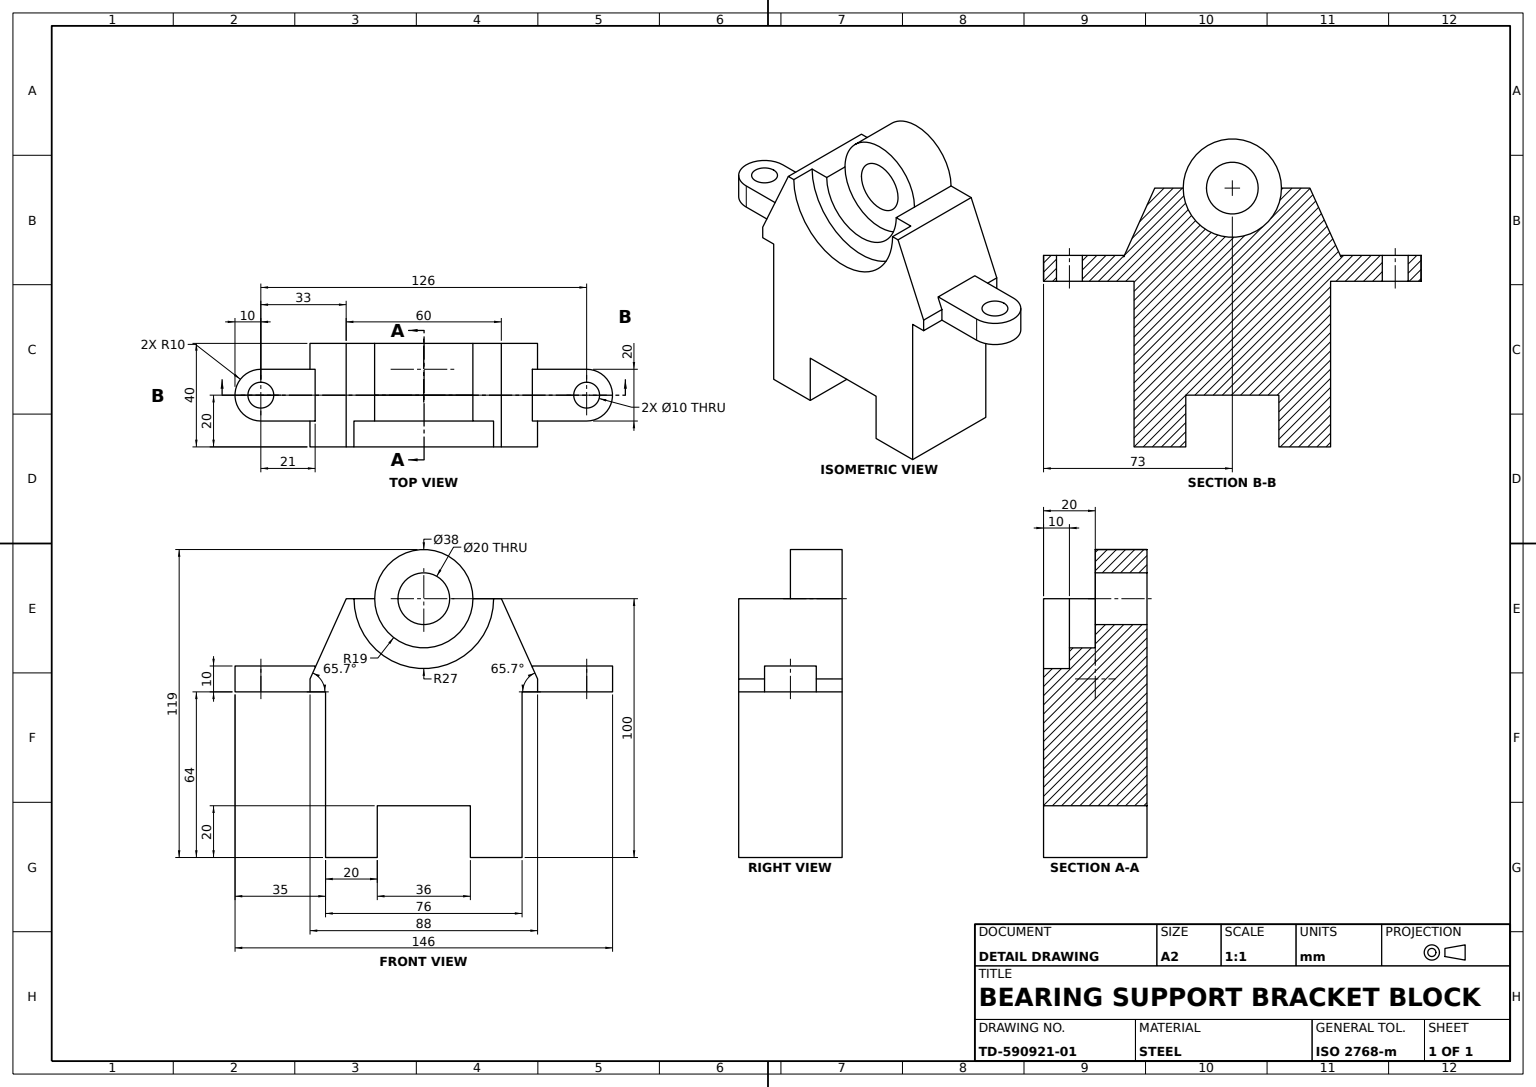
from build123d import *

# Parameters (mm, degrees)
BASE_BODY_DEPTH             = 40
UPPER_BODY_DEPTH            = 40
LEFT_LUG_BLOCK_SKETCH_W     = 20
LEFT_LUG_BLOCK_SKETCH_H     = 5
LEFT_LUG_BLOCK_DEPTH        = 19
LEFT_LUG_ARM_SKETCH_W       = 20
LEFT_LUG_ARM_SKETCH_H       = 5
LEFT_LUG_ARM_DEPTH          = 21
LEFT_LUG_ROUNDED_END_DEPTH  = 10
LEFT_LUG_HOLE_SKETCH_R      = 5
LEFT_LUG_HOLE_10_DEPTH      = 10
RIGHT_LUG_BLOCK_SKETCH_W    = 20
RIGHT_LUG_BLOCK_SKETCH_H    = 5
RIGHT_LUG_BLOCK_DEPTH       = 19
RIGHT_LUG_ARM_SKETCH_W      = 20
RIGHT_LUG_ARM_SKETCH_H      = 5
RIGHT_LUG_ARM_DEPTH         = 21
RIGHT_LUG_ROUNDED_END_DEPTH = 10
RIGHT_LUG_HOLE_SKETCH_R     = 5
RIGHT_LUG_HOLE_10_DEPTH     = 10
BEARING_SEAT_CUT_54_DEPTH   = 10
SEAT_GROOVE_38_DEPTH        = 30
HUB_SKETCH_R                = 19
HUB_38_DEPTH                = 30
HUB_RECESS_SKETCH_R         = 19
HUB_RECESS_38_DEPTH         = 10
BORE_SKETCH_R               = 10
BORE_20_DEPTH               = 20


with BuildPart() as part:
    # Base Body Sketch → Base Body (new body)
    with BuildSketch(Plane.XY):
        Polygon((0, 0), (0, 64), (76, 64), (76, 0), (56, 0), (56, 20), (20, 20), (20, 0), align=None)
    extrude(amount=BASE_BODY_DEPTH)

    # Upper Body Sketch → Upper Body (add)
    with BuildSketch(Plane.XY.offset(40)):
        Polygon((0, 64), (-6, 64), (-6, 69), (8, 100), (38, 100), (68, 100), (82, 69), (82, 64), (76, 64), align=None)
    extrude(amount=-UPPER_BODY_DEPTH)

    # Left Lug Block Sketch → Left Lug Block (add)
    with BuildSketch(Plane.ZY.offset(6)):
        with Locations((20, 66.5)):
            Rectangle(LEFT_LUG_BLOCK_SKETCH_W, LEFT_LUG_BLOCK_SKETCH_H)
    extrude(amount=LEFT_LUG_BLOCK_DEPTH)

    # Left Lug Arm Sketch → Left Lug Arm (add)
    with BuildSketch(Plane.ZY.offset(25)):
        with Locations((20, 71.5)):
            Rectangle(LEFT_LUG_ARM_SKETCH_W, LEFT_LUG_ARM_SKETCH_H)
    extrude(amount=-LEFT_LUG_ARM_DEPTH)

    # Left Lug End Sketch → Left Lug Rounded End (add)
    with BuildSketch(Plane(origin=(0, 74, 0), x_dir=(1, 0, 0), z_dir=(0, 1, 0))):
        with BuildLine():
            Line((-25, -10), (-25, -30))
            ThreePointArc((-25, -30), (-35, -20), (-25, -10))
        make_face()
    extrude(amount=-LEFT_LUG_ROUNDED_END_DEPTH)

    # Left Lug Hole Sketch → Left Lug Hole Ø10 (cut)
    with BuildSketch(Plane(origin=(0, 74, 0), x_dir=(1, 0, 0), z_dir=(0, 1, 0))):
        with Locations(Location((-25, -20, 0), (0, 0, 270))):
            Circle(LEFT_LUG_HOLE_SKETCH_R)
    extrude(amount=-LEFT_LUG_HOLE_10_DEPTH, mode=Mode.SUBTRACT)

    # Right Lug Block Sketch → Right Lug Block (add)
    with BuildSketch(Plane(origin=(82, 0, 0), x_dir=(0, 0, -1), z_dir=(1, 0, 0))):
        with Locations((-20, 66.5)):
            Rectangle(RIGHT_LUG_BLOCK_SKETCH_W, RIGHT_LUG_BLOCK_SKETCH_H)
    extrude(amount=RIGHT_LUG_BLOCK_DEPTH)

    # Right Lug Arm Sketch → Right Lug Arm (add)
    with BuildSketch(Plane(origin=(101, 0, 0), x_dir=(0, 0, -1), z_dir=(1, 0, 0))):
        with Locations((-20, 71.5)):
            Rectangle(RIGHT_LUG_ARM_SKETCH_W, RIGHT_LUG_ARM_SKETCH_H)
    extrude(amount=-RIGHT_LUG_ARM_DEPTH)

    # Right Lug End Sketch → Right Lug Rounded End (add)
    with BuildSketch(Plane(origin=(0, 74, 0), x_dir=(1, 0, 0), z_dir=(0, 1, 0))):
        with BuildLine():
            Line((101, -10), (101, -30))
            ThreePointArc((101, -30), (111, -20), (101, -10))
        make_face()
    extrude(amount=-RIGHT_LUG_ROUNDED_END_DEPTH)

    # Right Lug Hole Sketch → Right Lug Hole Ø10 (cut)
    with BuildSketch(Plane(origin=(0, 74, 0), x_dir=(1, 0, 0), z_dir=(0, 1, 0))):
        with Locations(Location((101, -20, 0), (0, 0, 270))):
            Circle(RIGHT_LUG_HOLE_SKETCH_R)
    extrude(amount=-RIGHT_LUG_HOLE_10_DEPTH, mode=Mode.SUBTRACT)

    # Bearing Seat Sketch → Bearing Seat Cut Ø54 (cut)
    with BuildSketch(Plane.XY.offset(40)):
        with BuildLine():
            Line((11, 100), (65, 100))
            ThreePointArc((65, 100), (38, 73), (11, 100))
        make_face()
    extrude(amount=-BEARING_SEAT_CUT_54_DEPTH, mode=Mode.SUBTRACT)

    # Seat Groove Sketch → Seat Groove Ø38 (cut)
    with BuildSketch(Plane.XY.offset(30)):
        with BuildLine():
            Line((19, 100), (57, 100))
            ThreePointArc((57, 100), (38, 81), (19, 100))
        make_face()
    extrude(amount=-SEAT_GROOVE_38_DEPTH, mode=Mode.SUBTRACT)

    # Hub Sketch → Hub Ø38 (add)
    with BuildSketch(Plane.XY.offset(30)):
        with Locations((38, 100)):
            Circle(HUB_SKETCH_R)
    extrude(amount=-HUB_38_DEPTH)

    # Hub Recess Sketch → Hub Recess Ø38 (cut)
    with BuildSketch(Plane.XY.offset(30)):
        with Locations((38, 100)):
            Circle(HUB_RECESS_SKETCH_R)
    extrude(amount=-HUB_RECESS_38_DEPTH, mode=Mode.SUBTRACT)

    # Bore Sketch → Bore Ø20 (cut)
    with BuildSketch(Plane.XY.offset(20)):
        with Locations((38, 100)):
            Circle(BORE_SKETCH_R)
    extrude(amount=-BORE_20_DEPTH, mode=Mode.SUBTRACT)


solid = part.part
